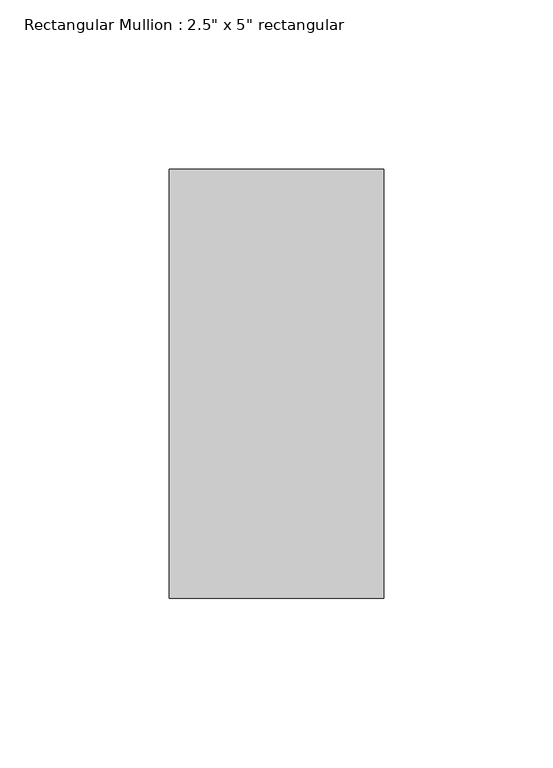
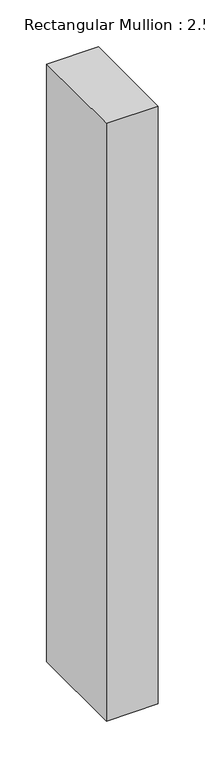
"""IFC4 building model written with IfcOpenShell, lengths in millimetres: member geometry."""

from ifc_helpers import new_model, si_unit, frame, origin, place, context, project, spatial, polyline, outline, extrude, source, transform, mapped, element, save


def member_53377e5f(model_context):
    return source(origin(), model_context, "Body", "SweptSolid", [
        extrude(outline(polyline([(0.0, 63.5), (0.0, -63.5), (-63.5, -63.5), (-63.5, 63.5), (0.0, 63.5)])), frame((0.0, 0.0, -777.2877103), z_axis=(0.0, 0.0, 1.0), x_axis=(1.0, 0.0, 0.0)), (0.0, 0.0, 1.0), 777.2877103),
    ])


if __name__ == "__main__":
    model = new_model("IFC4")
    model_context = context("Model", 3, world=origin())
    ifc_project = project(units=[si_unit("LENGTHUNIT", "METRE", prefix="MILLI")], contexts=[model_context])
    site = spatial("IfcSite", under=ifc_project)
    building = spatial("IfcBuilding", under=site)
    placement = place(None, origin())
    member_shape = member_53377e5f(model_context)
    element("IfcMember", 1, ObjectType="Rectangular Mullion : 2.5\" x 5\" rectangular", at=placement, inside=building, context=model_context, shape_type="MappedRepresentation", body=[
        mapped(member_shape, transform((0.0, 0.0, 0.0), x_axis=(1.0, 0.0, 0.0), y_axis=(0.0, 1.0, 0.0), z_axis=(0.0, 0.0, 1.0))),
    ])
    save(model, "model.ifc")

# Revit data of these elements
# Type "Rectangular Mullion : 2.5\" x 5\" rectangular"
#   built-in parameter 1007304 = 0.416667 (stored number, unit not read)
#   built-in parameter 1007301 = 0.104167 (stored number, unit not read)
#   built-in parameter 1007300 = 0.104167 (stored number, unit not read)
# Element 1 (IfcMember, "Rectangular Mullion : 2.5\" x 5\" rectangular")
#   Materials on its faces: "Aluminum"
# Materials
#   "Aluminum": class "Metal", colour RGB 247 247 247, transparency 0, Description = "Aluminum 6061", Cost = 0
